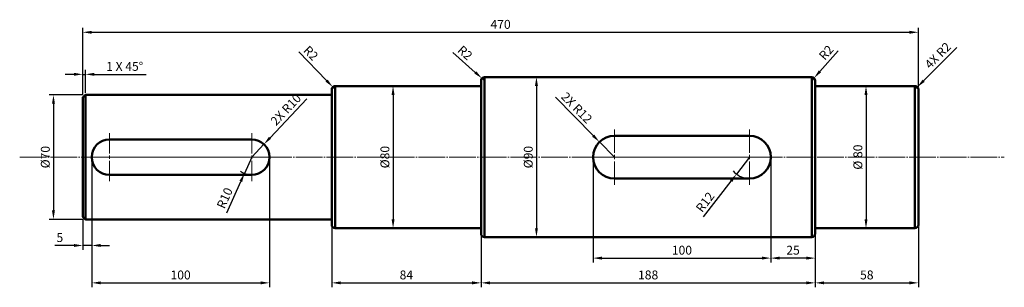
# Model space of a CAD drawing. Units: millimetres. Extents: x 186344 to 186897, y 72203 to 72353.
import ezdxf

# ---------------------------------------------------------------- set-up
doc = ezdxf.new("R2010")
doc.units = ezdxf.units.MM
doc.linetypes.add('HIDDENX2', pattern=[19.05, 12.7, -6.35])
doc.linetypes.add('JIS_08_15', pattern=[17.25, 15, -0.75, 0.75, -0.75])
doc.layers.get('Defpoints').update_dxf_attribs({"color": 3, "linetype": 'HIDDENX2'})
for name, color, linetype, lineweight in [('M-CNTR', 1, 'JIS_08_15', 18), ('M-DIMS', 4, 'Continuous', 25), ('M-OUTL', 7, 'Continuous', 50)]:
    doc.layers.add(name, color=color, linetype=linetype, lineweight=lineweight)
doc.styles.add('Annotative', font='arial.ttf')
doc.styles.get("Standard").update_dxf_attribs({"font": 'arial.ttf'})
doc.dimstyles.new('ISO-25', dxfattribs={"dimscale": 2, "dimtxt": 2.5, "dimasz": 2.5, "dimexe": 1.25, "dimexo": 0.625, "dimtad": 1, "dimtxsty": 'Standard', "dimcen": 2.5, "dimadec": 0, "dimazin": 0, "dimtfac": 1, "dimtmove": 0, "dimatfit": 3, "dimfxl": 1, "dimarcsym": 0})

# ---------------------------------------------------------------- blocks, each defined once
blk = doc.blocks.new('*U1')
at = {"layer": 'M-CNTR', "color": 0, "transparency": 16777216}
for p, q in [((0, 2.4), (0, 15.5)), ((-15.5, 0), (-2.4, 0)), ((2.4, 0), (15.5, 0)), ((0, -15.5), (0, -2.4))]:
    blk.add_line(p, q, dxfattribs=at)
at = {"layer": 'M-CNTR', "color": 0, "linetype": 'Continuous', "transparency": 16777216}
for p, q in [((-1.2, 0), (1.2, 0)), ((0, -1.2), (0, 1.2))]:
    blk.add_line(p, q, dxfattribs=at)
blk = doc.blocks.new('*U2')
at = {"layer": 'M-CNTR', "color": 0, "transparency": 16777216}
for p, q in [((0, 2.4), (0, 15.5)), ((-15.5, 0), (-2.4, 0)), ((2.4, 0), (15.5, 0)), ((0, -15.5), (0, -2.4))]:
    blk.add_line(p, q, dxfattribs=at)
at = {"layer": 'M-CNTR', "color": 0, "linetype": 'Continuous', "transparency": 16777216}
for p, q in [((-1.2, 0), (1.2, 0)), ((0, -1.2), (0, 1.2))]:
    blk.add_line(p, q, dxfattribs=at)
blk = doc.blocks.new('*D10')
at = {"layer": 'Defpoints', "color": 0, "transparency": 16777216}
for p in [(186380.52, 72311.16), (186362.58, 72241.16), (186380.52, 72241.16)]:
    blk.add_point(p, dxfattribs=at)
at = {"layer": 'M-DIMS', "color": 0, "lineweight": -2, "transparency": 16777216}
for p, q in [((186379.27, 72311.16), (186360.08, 72311.16)), ((186362.58, 72306.16), (186362.58, 72246.16)), ((186379.27, 72241.16), (186360.08, 72241.16))]:
    blk.add_line(p, q, dxfattribs=at)
at = {"layer": 'M-DIMS', "color": 0, "transparency": 16777216}
for points in [[(186361.75, 72306.16), (186363.42, 72306.16), (186362.58, 72311.16)], [(186361.75, 72246.16), (186363.42, 72246.16), (186362.58, 72241.16)]]:
    blk.add_solid(points, dxfattribs=at)
at = {"layer": 'M-DIMS', "color": 0, "transparency": 16777216, "insert": (186358.64, 72276.16), "char_height": 5, "attachment_point": 5, "rotation": 90, "style": 'Annotative'}
blk.add_mtext('%%C70', dxfattribs=at)
blk = doc.blocks.new('*D11')
at = {"layer": 'Defpoints', "color": 0, "transparency": 16777216}
for p in [(186549.8, 72316.16), (186549.8, 72236.16), (186553.62, 72236.16)]:
    blk.add_point(p, dxfattribs=at)
at = {"layer": 'M-DIMS', "color": 0, "lineweight": -2, "transparency": 16777216}
for p, q in [((186551.05, 72316.16), (186556.12, 72316.16)), ((186553.62, 72311.16), (186553.62, 72241.16)), ((186551.05, 72236.16), (186556.12, 72236.16))]:
    blk.add_line(p, q, dxfattribs=at)
at = {"layer": 'M-DIMS', "color": 0, "transparency": 16777216}
for points in [[(186552.79, 72311.16), (186554.46, 72311.16), (186553.62, 72316.16)], [(186552.79, 72241.16), (186554.46, 72241.16), (186553.62, 72236.16)]]:
    blk.add_solid(points, dxfattribs=at)
at = {"layer": 'M-DIMS', "color": 0, "transparency": 16777216, "insert": (186549.68, 72276.16), "char_height": 5, "attachment_point": 5, "rotation": 90, "style": 'Annotative'}
blk.add_mtext('%%C80', dxfattribs=at)
blk = doc.blocks.new('*D12')
at = {"layer": 'Defpoints', "color": 0, "transparency": 16777216}
for p in [(186639.08, 72321.16), (186634.27, 72231.16), (186639.08, 72231.16)]:
    blk.add_point(p, dxfattribs=at)
at = {"layer": 'M-DIMS', "color": 0, "lineweight": -2, "transparency": 16777216}
for p, q in [((186637.83, 72321.16), (186631.77, 72321.16)), ((186634.27, 72316.16), (186634.27, 72236.16)), ((186637.83, 72231.16), (186631.77, 72231.16))]:
    blk.add_line(p, q, dxfattribs=at)
at = {"layer": 'M-DIMS', "color": 0, "transparency": 16777216}
for points in [[(186633.43, 72316.16), (186635.1, 72316.16), (186634.27, 72321.16)], [(186633.43, 72236.16), (186635.1, 72236.16), (186634.27, 72231.16)]]:
    blk.add_solid(points, dxfattribs=at)
at = {"layer": 'M-DIMS', "color": 0, "transparency": 16777216, "insert": (186630.32, 72276.16), "char_height": 5, "attachment_point": 5, "rotation": 90, "style": 'Annotative'}
blk.add_mtext('%%C90', dxfattribs=at)
blk = doc.blocks.new('*D13')
at = {"layer": 'Defpoints', "color": 0, "transparency": 16777216}
for p in [(186813.24, 72316.16), (186813.24, 72236.16), (186819.65, 72236.16)]:
    blk.add_point(p, dxfattribs=at)
at = {"layer": 'M-DIMS', "color": 0, "lineweight": -2, "transparency": 16777216}
for p, q in [((186814.49, 72316.16), (186822.15, 72316.16)), ((186819.65, 72311.16), (186819.65, 72241.16)), ((186814.49, 72236.16), (186822.15, 72236.16))]:
    blk.add_line(p, q, dxfattribs=at)
at = {"layer": 'M-DIMS', "color": 0, "transparency": 16777216}
for points in [[(186818.82, 72311.16), (186820.49, 72311.16), (186819.65, 72316.16)], [(186818.82, 72241.16), (186820.49, 72241.16), (186819.65, 72236.16)]]:
    blk.add_solid(points, dxfattribs=at)
at = {"layer": 'M-DIMS', "color": 0, "transparency": 16777216, "insert": (186815.71, 72276.16), "char_height": 5, "attachment_point": 5, "rotation": 90, "style": 'Annotative'}
blk.add_mtext('%%C 80', dxfattribs=at)
blk = doc.blocks.new('*D14')
at = {"layer": 'Defpoints', "color": 0, "transparency": 16777216}
for p in [(186380.52, 72322.73), (186379.1, 72309.75), (186380.52, 72311.16)]:
    blk.add_point(p, dxfattribs=at)
at = {"layer": 'M-DIMS', "color": 0, "lineweight": -2, "transparency": 16777216}
for p, q in [((186374.1, 72322.73), (186369.1, 72322.73)), ((186379.1, 72311), (186379.1, 72325.23)), ((186379.1, 72322.73), (186380.52, 72322.73)), ((186380.52, 72312.41), (186380.52, 72325.23)), ((186385.52, 72322.73), (186414.78, 72322.73))]:
    blk.add_line(p, q, dxfattribs=at)
at = {"layer": 'M-DIMS', "color": 0, "transparency": 16777216}
for points in [[(186374.1, 72323.57), (186374.1, 72321.9), (186379.1, 72322.73)], [(186385.52, 72323.57), (186385.52, 72321.9), (186380.52, 72322.73)]]:
    blk.add_solid(points, dxfattribs=at)
at = {"layer": 'M-DIMS', "color": 0, "transparency": 16777216, "insert": (186402.65, 72326.54), "char_height": 5, "attachment_point": 5, "style": 'Annotative'}
blk.add_mtext('1 X 45%%D', dxfattribs=at)
blk = doc.blocks.new('*U3')
at = {"layer": 'M-CNTR', "color": 0, "transparency": 16777216}
for p, q in [((0, 2), (0, 13.5)), ((-13.5, 0), (-2, 0)), ((2, 0), (13.5, 0)), ((0, -13.5), (0, -2))]:
    blk.add_line(p, q, dxfattribs=at)
at = {"layer": 'M-CNTR', "color": 0, "linetype": 'Continuous', "transparency": 16777216}
for p, q in [((-1, 0), (1, 0)), ((0, -1), (0, 1))]:
    blk.add_line(p, q, dxfattribs=at)
blk = doc.blocks.new('*U4')
at = {"layer": 'M-CNTR', "color": 0, "transparency": 16777216}
for p, q in [((0, 2), (0, 13.5)), ((-13.5, 0), (-2, 0)), ((2, 0), (13.5, 0)), ((0, -13.5), (0, -2))]:
    blk.add_line(p, q, dxfattribs=at)
at = {"layer": 'M-CNTR', "color": 0, "linetype": 'Continuous', "transparency": 16777216}
for p, q in [((-1, 0), (1, 0)), ((0, -1), (0, 1))]:
    blk.add_line(p, q, dxfattribs=at)
blk = doc.blocks.new('*D5')
at = {"layer": 'Defpoints', "color": 0, "transparency": 16777216}
for p in [(186474.1, 72276.16), (186470.01, 72267.03)]:
    blk.add_point(p, dxfattribs=at)
at = {"layer": 'M-DIMS', "color": 0, "lineweight": -2, "transparency": 16777216}
for p, q in [((186474.1, 72276.16), (186470.01, 72267.03)), ((186460.02, 72244.74), (186467.97, 72262.47))]:
    blk.add_line(p, q, dxfattribs=at)
blk.add_arc((186474.1, 72276.16), 10, 231.532, 262.838, dxfattribs=at)
at = {"layer": 'M-DIMS', "color": 0, "transparency": 16777216}
blk.add_solid([(186467.21, 72262.81), (186468.73, 72262.13), (186470.01, 72267.03)], dxfattribs=at)
at = {"layer": 'M-DIMS', "color": 0, "transparency": 16777216, "insert": (186459.5, 72252.88), "char_height": 5, "attachment_point": 5, "rotation": 65.856, "style": 'Annotative'}
blk.add_mtext('R10', dxfattribs=at)
blk = doc.blocks.new('*D6')
at = {"layer": 'Defpoints', "color": 0, "transparency": 16777216}
for p in [(186754.1, 72276.16), (186746.79, 72266.64)]:
    blk.add_point(p, dxfattribs=at)
at = {"layer": 'M-DIMS', "color": 0, "lineweight": -2, "transparency": 16777216}
for p, q in [((186754.1, 72276.16), (186746.79, 72266.64)), ((186728.23, 72242.49), (186743.74, 72262.68))]:
    blk.add_line(p, q, dxfattribs=at)
blk.add_arc((186754.1, 72276.16), 12, 220.5254, 264.0317, dxfattribs=at)
at = {"layer": 'M-DIMS', "color": 0, "transparency": 16777216}
blk.add_solid([(186743.08, 72263.19), (186744.41, 72262.17), (186746.79, 72266.64)], dxfattribs=at)
at = {"layer": 'M-DIMS', "color": 0, "transparency": 16777216, "insert": (186729.63, 72250.48), "char_height": 5, "attachment_point": 5, "rotation": 52.462, "style": 'Annotative'}
blk.add_mtext('R12', dxfattribs=at)
blk = doc.blocks.new('*D7')
at = {"layer": 'Defpoints', "color": 0, "transparency": 16777216}
for p in [(186519.71, 72315.6), (186521.1, 72314.16)]:
    blk.add_point(p, dxfattribs=at)
at = {"layer": 'M-DIMS', "color": 0, "lineweight": -2, "transparency": 16777216}
for p, q in [((186500.56, 72335.36), (186516.23, 72319.19)), ((186521.1, 72314.16), (186519.71, 72315.6))]:
    blk.add_line(p, q, dxfattribs=at)
at = {"layer": 'M-DIMS', "color": 0, "transparency": 16777216}
blk.add_solid([(186516.83, 72319.77), (186515.63, 72318.61), (186519.71, 72315.6)], dxfattribs=at)
at = {"layer": 'M-DIMS', "color": 0, "transparency": 16777216, "insert": (186506.92, 72334.2), "char_height": 5, "attachment_point": 5, "rotation": 314.0907, "style": 'Annotative'}
blk.add_mtext('R2', dxfattribs=at)
blk = doc.blocks.new('*D8')
at = {"layer": 'Defpoints', "color": 0, "transparency": 16777216}
for p in [(186603.61, 72320.49), (186605.1, 72319.16)]:
    blk.add_point(p, dxfattribs=at)
at = {"layer": 'M-DIMS', "color": 0, "lineweight": -2, "transparency": 16777216}
for p, q in [((186587.26, 72335.07), (186599.88, 72323.82)), ((186605.1, 72319.16), (186603.61, 72320.49))]:
    blk.add_line(p, q, dxfattribs=at)
at = {"layer": 'M-DIMS', "color": 0, "transparency": 16777216}
blk.add_solid([(186600.43, 72324.44), (186599.32, 72323.2), (186603.61, 72320.49)], dxfattribs=at)
at = {"layer": 'M-DIMS', "color": 0, "transparency": 16777216, "insert": (186593.68, 72334.38), "char_height": 5, "attachment_point": 5, "rotation": 318.2831, "style": 'Annotative'}
blk.add_mtext('R2', dxfattribs=at)
blk = doc.blocks.new('*D9')
at = {"layer": 'Defpoints', "color": 0, "transparency": 16777216}
for p in [(186789.1, 72319.16), (186790.43, 72320.66)]:
    blk.add_point(p, dxfattribs=at)
at = {"layer": 'M-DIMS', "color": 0, "lineweight": -2, "transparency": 16777216}
for p, q in [((186804.03, 72336.01), (186793.74, 72324.4)), ((186789.1, 72319.16), (186790.43, 72320.66))]:
    blk.add_line(p, q, dxfattribs=at)
at = {"layer": 'M-DIMS', "color": 0, "transparency": 16777216}
blk.add_solid([(186793.12, 72324.95), (186794.37, 72323.85), (186790.43, 72320.66)], dxfattribs=at)
at = {"layer": 'M-DIMS', "color": 0, "transparency": 16777216, "insert": (186797.73, 72334.57), "char_height": 5, "attachment_point": 5, "rotation": 48.4635, "style": 'Annotative'}
blk.add_mtext('R2', dxfattribs=at)
blk = doc.blocks.new('*D15')
at = {"layer": 'Defpoints', "color": 0, "transparency": 16777216}
for p in [(186384.1, 72276.16), (186379.1, 72242.57), (186379.1, 72226.46)]:
    blk.add_point(p, dxfattribs=at)
at = {"layer": 'M-DIMS', "color": 0, "lineweight": -2, "transparency": 16777216}
for p, q in [((186384.1, 72274.91), (186384.1, 72223.96)), ((186379.1, 72241.32), (186379.1, 72223.96)), ((186374.1, 72226.46), (186363.29, 72226.46)), ((186384.1, 72226.46), (186379.1, 72226.46)), ((186389.1, 72226.46), (186394.1, 72226.46))]:
    blk.add_line(p, q, dxfattribs=at)
at = {"layer": 'M-DIMS', "color": 0, "transparency": 16777216}
for points in [[(186374.1, 72227.3), (186374.1, 72225.63), (186379.1, 72226.46)], [(186389.1, 72227.3), (186389.1, 72225.63), (186384.1, 72226.46)]]:
    blk.add_solid(points, dxfattribs=at)
at = {"layer": 'M-DIMS', "color": 0, "transparency": 16777216, "insert": (186366.19, 72230.26), "char_height": 5, "attachment_point": 5, "style": 'Annotative'}
blk.add_mtext('5', dxfattribs=at)
blk = doc.blocks.new('*D16')
at = {"layer": 'Defpoints', "color": 0, "transparency": 16777216}
for p in [(186384.1, 72276.16), (186484.1, 72276.16), (186484.1, 72205.43)]:
    blk.add_point(p, dxfattribs=at)
at = {"layer": 'M-DIMS', "color": 0, "lineweight": -2, "transparency": 16777216}
for p, q in [((186384.1, 72274.91), (186384.1, 72202.93)), ((186484.1, 72274.91), (186484.1, 72202.93)), ((186389.1, 72205.43), (186479.1, 72205.43))]:
    blk.add_line(p, q, dxfattribs=at)
at = {"layer": 'M-DIMS', "color": 0, "transparency": 16777216}
for points in [[(186389.1, 72206.26), (186389.1, 72204.59), (186384.1, 72205.43)], [(186479.1, 72206.26), (186479.1, 72204.59), (186484.1, 72205.43)]]:
    blk.add_solid(points, dxfattribs=at)
at = {"layer": 'M-DIMS', "color": 0, "transparency": 16777216, "insert": (186434.1, 72209.23), "char_height": 5, "attachment_point": 5, "style": 'Annotative'}
blk.add_mtext('100', dxfattribs=at)
blk = doc.blocks.new('*D17')
at = {"layer": 'Defpoints', "color": 0, "transparency": 16777216}
for p in [(186519.1, 72241.16), (186603.1, 72236.16), (186603.1, 72205.43)]:
    blk.add_point(p, dxfattribs=at)
at = {"layer": 'M-DIMS', "color": 0, "lineweight": -2, "transparency": 16777216}
for p, q in [((186519.1, 72239.91), (186519.1, 72202.93)), ((186603.1, 72234.91), (186603.1, 72202.93)), ((186524.1, 72205.43), (186598.1, 72205.43))]:
    blk.add_line(p, q, dxfattribs=at)
at = {"layer": 'M-DIMS', "color": 0, "transparency": 16777216}
for points in [[(186524.1, 72206.26), (186524.1, 72204.59), (186519.1, 72205.43)], [(186598.1, 72206.26), (186598.1, 72204.59), (186603.1, 72205.43)]]:
    blk.add_solid(points, dxfattribs=at)
at = {"layer": 'M-DIMS', "color": 0, "transparency": 16777216, "insert": (186561.1, 72209.23), "char_height": 5, "attachment_point": 5, "style": 'Annotative'}
blk.add_mtext('84', dxfattribs=at)
blk = doc.blocks.new('*D18')
at = {"layer": 'Defpoints', "color": 0, "transparency": 16777216}
for p in [(186603.1, 72236.16), (186791.1, 72236.16), (186791.1, 72205.43)]:
    blk.add_point(p, dxfattribs=at)
at = {"layer": 'M-DIMS', "color": 0, "lineweight": -2, "transparency": 16777216}
for p, q in [((186603.1, 72234.91), (186603.1, 72202.93)), ((186791.1, 72234.91), (186791.1, 72202.93)), ((186608.1, 72205.43), (186786.1, 72205.43))]:
    blk.add_line(p, q, dxfattribs=at)
at = {"layer": 'M-DIMS', "color": 0, "transparency": 16777216}
for points in [[(186608.1, 72206.26), (186608.1, 72204.59), (186603.1, 72205.43)], [(186786.1, 72206.26), (186786.1, 72204.59), (186791.1, 72205.43)]]:
    blk.add_solid(points, dxfattribs=at)
at = {"layer": 'M-DIMS', "color": 0, "transparency": 16777216, "insert": (186697.1, 72209.23), "char_height": 5, "attachment_point": 5, "style": 'Annotative'}
blk.add_mtext('188', dxfattribs=at)
blk = doc.blocks.new('*D19')
at = {"layer": 'Defpoints', "color": 0, "transparency": 16777216}
for p in [(186791.1, 72236.16), (186849.1, 72238.16), (186849.1, 72205.43)]:
    blk.add_point(p, dxfattribs=at)
at = {"layer": 'M-DIMS', "color": 0, "lineweight": -2, "transparency": 16777216}
for p, q in [((186791.1, 72234.91), (186791.1, 72202.93)), ((186849.1, 72236.91), (186849.1, 72202.93)), ((186796.1, 72205.43), (186844.1, 72205.43))]:
    blk.add_line(p, q, dxfattribs=at)
at = {"layer": 'M-DIMS', "color": 0, "transparency": 16777216}
for points in [[(186796.1, 72206.26), (186796.1, 72204.59), (186791.1, 72205.43)], [(186844.1, 72206.26), (186844.1, 72204.59), (186849.1, 72205.43)]]:
    blk.add_solid(points, dxfattribs=at)
at = {"layer": 'M-DIMS', "color": 0, "transparency": 16777216, "insert": (186820.1, 72209.23), "char_height": 5, "attachment_point": 5, "style": 'Annotative'}
blk.add_mtext('58', dxfattribs=at)
blk = doc.blocks.new('*D20')
at = {"layer": 'Defpoints', "color": 0, "transparency": 16777216}
for p in [(186766.1, 72276.16), (186791.1, 72236.16), (186766.1, 72219.35)]:
    blk.add_point(p, dxfattribs=at)
at = {"layer": 'M-DIMS', "color": 0, "lineweight": -2, "transparency": 16777216}
for p, q in [((186766.1, 72274.91), (186766.1, 72216.85)), ((186791.1, 72234.91), (186791.1, 72216.85)), ((186786.1, 72219.35), (186771.1, 72219.35))]:
    blk.add_line(p, q, dxfattribs=at)
at = {"layer": 'M-DIMS', "color": 0, "transparency": 16777216}
for points in [[(186771.1, 72220.19), (186771.1, 72218.52), (186766.1, 72219.35)], [(186786.1, 72220.19), (186786.1, 72218.52), (186791.1, 72219.35)]]:
    blk.add_solid(points, dxfattribs=at)
at = {"layer": 'M-DIMS', "color": 0, "transparency": 16777216, "insert": (186778.6, 72223.16), "char_height": 5, "attachment_point": 5, "style": 'Annotative'}
blk.add_mtext('25', dxfattribs=at)
blk = doc.blocks.new('*D21')
at = {"layer": 'Defpoints', "color": 0, "transparency": 16777216}
for p in [(186666.1, 72276.16), (186766.1, 72276.16), (186766.1, 72219.35)]:
    blk.add_point(p, dxfattribs=at)
at = {"layer": 'M-DIMS', "color": 0, "lineweight": -2, "transparency": 16777216}
for p, q in [((186666.1, 72274.91), (186666.1, 72216.85)), ((186766.1, 72274.91), (186766.1, 72216.85)), ((186671.1, 72219.35), (186761.1, 72219.35))]:
    blk.add_line(p, q, dxfattribs=at)
at = {"layer": 'M-DIMS', "color": 0, "transparency": 16777216}
for points in [[(186671.1, 72220.19), (186671.1, 72218.52), (186666.1, 72219.35)], [(186761.1, 72220.19), (186761.1, 72218.52), (186766.1, 72219.35)]]:
    blk.add_solid(points, dxfattribs=at)
at = {"layer": 'M-DIMS', "color": 0, "transparency": 16777216, "insert": (186716.1, 72223.16), "char_height": 5, "attachment_point": 5, "style": 'Annotative'}
blk.add_mtext('100', dxfattribs=at)
blk = doc.blocks.new('*D22')
at = {"layer": 'Defpoints', "color": 0, "transparency": 16777216}
for p in [(186849.1, 72346.39), (186849.1, 72314.16), (186379.1, 72309.75)]:
    blk.add_point(p, dxfattribs=at)
at = {"layer": 'M-DIMS', "color": 0, "lineweight": -2, "transparency": 16777216}
for p, q in [((186379.1, 72311), (186379.1, 72348.89)), ((186384.1, 72346.39), (186844.1, 72346.39)), ((186849.1, 72315.41), (186849.1, 72348.89))]:
    blk.add_line(p, q, dxfattribs=at)
at = {"layer": 'M-DIMS', "color": 0, "transparency": 16777216}
for points in [[(186384.1, 72347.22), (186384.1, 72345.55), (186379.1, 72346.39)], [(186844.1, 72347.22), (186844.1, 72345.55), (186849.1, 72346.39)]]:
    blk.add_solid(points, dxfattribs=at)
at = {"layer": 'M-DIMS', "color": 0, "transparency": 16777216, "insert": (186614.1, 72350.19), "char_height": 5, "attachment_point": 5, "style": 'Annotative'}
blk.add_mtext('470', dxfattribs=at)
blk = doc.blocks.new('*D23')
at = {"layer": 'Defpoints', "color": 0, "transparency": 16777216}
for p in [(186480.97, 72283.42), (186474.1, 72276.16)]:
    blk.add_point(p, dxfattribs=at)
at = {"layer": 'M-DIMS', "color": 0, "lineweight": -2, "transparency": 16777216}
for p, q in [((186505.2, 72309.04), (186484.41, 72287.06)), ((186474.1, 72276.16), (186480.97, 72283.42))]:
    blk.add_line(p, q, dxfattribs=at)
at = {"layer": 'M-DIMS', "color": 0, "transparency": 16777216}
blk.add_solid([(186483.8, 72287.63), (186485.02, 72286.48), (186480.97, 72283.42)], dxfattribs=at)
at = {"layer": 'M-DIMS', "color": 0, "transparency": 16777216, "insert": (186493.76, 72302.48), "char_height": 5, "attachment_point": 5, "rotation": 46.5937}
blk.add_mtext('2X R10', dxfattribs=at)
blk = doc.blocks.new('*D24')
at = {"layer": 'Defpoints', "color": 0, "transparency": 16777216}
for p in [(186669.68, 72284.71), (186678.1, 72276.16)]:
    blk.add_point(p, dxfattribs=at)
at = {"layer": 'M-DIMS', "color": 0, "lineweight": -2, "transparency": 16777216}
for p, q in [((186644.96, 72309.8), (186666.17, 72288.27)), ((186678.1, 72276.16), (186669.68, 72284.71))]:
    blk.add_line(p, q, dxfattribs=at)
at = {"layer": 'M-DIMS', "color": 0, "transparency": 16777216}
blk.add_solid([(186666.77, 72288.85), (186665.58, 72287.68), (186669.68, 72284.71)], dxfattribs=at)
at = {"layer": 'M-DIMS', "color": 0, "transparency": 16777216, "insert": (186656.49, 72303.46), "char_height": 5, "attachment_point": 5, "rotation": 314.5722}
blk.add_mtext('2X R12', dxfattribs=at)
blk = doc.blocks.new('*D25')
at = {"layer": 'Defpoints', "color": 0, "transparency": 16777216}
for p in [(186847.1, 72314.16), (186848.52, 72315.57)]:
    blk.add_point(p, dxfattribs=at)
at = {"layer": 'M-DIMS', "color": 0, "lineweight": -2, "transparency": 16777216}
for p, q in [((186870.76, 72337.82), (186852.05, 72319.11)), ((186847.1, 72314.16), (186848.52, 72315.57))]:
    blk.add_line(p, q, dxfattribs=at)
at = {"layer": 'M-DIMS', "color": 0, "transparency": 16777216}
blk.add_solid([(186851.46, 72319.7), (186852.64, 72318.52), (186848.52, 72315.57)], dxfattribs=at)
at = {"layer": 'M-DIMS', "color": 0, "transparency": 16777216, "insert": (186860.51, 72332.89), "char_height": 5, "attachment_point": 5, "rotation": 45.0017}
blk.add_mtext('4X R2', dxfattribs=at)

msp = doc.modelspace()

# ---------------------------------------------------------------- linework, layer by layer
at = {"layer": 'M-CNTR'}
for p, q in [((186343.59, 72276.159), (186897.446, 72276.159)), ((186384.102, 72276.159), (186484.102, 72276.159)), ((186659.11, 72276.159), (186771.465, 72276.159))]:
    msp.add_line(p, q, dxfattribs=at)
at = {"layer": 'M-OUTL'}
for p, q in [((186603.102, 72233.159), (186603.102, 72319.159)), ((186605.102, 72321.159), (186789.102, 72321.159)), ((186605.102, 72231.159), (186605.102, 72321.159)), ((186789.102, 72321.159), (186789.102, 72231.159)), ((186789.102, 72231.159), (186789.102, 72321.159)), ((186791.102, 72233.159), (186791.102, 72319.159)), ((186519.102, 72238.159), (186519.102, 72314.159)), ((186521.102, 72316.159), (186603.102, 72316.159)), ((186521.102, 72236.159), (186521.102, 72316.159)), ((186603.102, 72316.159), (186603.102, 72236.159)), ((186791.102, 72316.159), (186847.102, 72316.159)), ((186791.102, 72236.159), (186791.102, 72316.159)), ((186847.102, 72316.159), (186847.102, 72236.159)), ((186849.102, 72314.159), (186849.102, 72238.159)), ((186394.102, 72286.159), (186474.102, 72286.159)), ((186678.102, 72288.159), (186754.102, 72288.159)), ((186474.102, 72266.159), (186394.102, 72266.159)), ((186678.102, 72264.159), (186754.102, 72264.159)), ((186603.102, 72236.159), (186521.102, 72236.159)), ((186847.102, 72236.159), (186791.102, 72236.159)), ((186789.102, 72231.159), (186605.102, 72231.159))]:
    msp.add_line(p, q, dxfattribs=at)
msp.add_lwpolyline([(186380.517, 72241.159), (186379.102, 72242.573), (186379.102, 72309.745), (186380.517, 72311.159), (186380.517, 72241.159), (186519.102, 72241.159), (186519.102, 72311.159), (186380.517, 72311.159)], dxfattribs=at)
for centre, radius, start, end in [((186605.102, 72319.159), 2, 90, 180), ((186789.102, 72319.159), 2, 0, 90), ((186521.102, 72314.159), 2, 90, 180), ((186847.102, 72314.159), 2, 0, 90), ((186394.102, 72276.159), 10, 90, 270), ((186474.102, 72276.159), 10, 270, 90), ((186678.102, 72276.159), 12, 90, 270), ((186754.102, 72276.159), 12, 270, 90), ((186521.102, 72238.159), 2, 180, 270), ((186847.102, 72238.159), 2, 270, 0), ((186605.102, 72233.159), 2, 180, 270), ((186789.102, 72233.159), 2, 270, 0)]:
    msp.add_arc(centre, radius, start, end, dxfattribs=at)

# ---------------------------------------------------------------- block references
at = {"layer": 'M-CNTR'}
for name, p in [('*U3', (186394.102, 72276.159)), ('*U4', (186474.102, 72276.159)), ('*U1', (186678.102, 72276.159)), ('*U2', (186754.102, 72276.159))]:
    msp.add_blockref(name, p, dxfattribs=at)

# ---------------------------------------------------------------- dimensions: what is measured, and where the dimension line sits
at = {"layer": 'M-DIMS'}
for base, p1, p2, picture, middle in [((186849.102, 72346.385), (186379.102, 72309.745), (186849.102, 72314.159), '*D22', (186614.102, 72350.188)), ((186379.102, 72226.463), (186384.102, 72276.159), (186379.102, 72242.573), '*D15', (186366.195, 72230.256)), ((186484.102, 72205.426), (186384.102, 72276.159), (186484.102, 72276.159), '*D16', (186434.102, 72209.229)), ((186766.102, 72219.354), (186666.102, 72276.159), (186766.102, 72276.159), '*D21', (186716.102, 72223.157)), ((186766.102, 72219.354), (186791.102, 72236.159), (186766.102, 72276.159), '*D20', (186778.602, 72223.157)), ((186603.102, 72205.426), (186519.102, 72241.159), (186603.102, 72236.159), '*D17', (186561.102, 72209.229)), ((186791.102, 72205.426), (186603.102, 72236.159), (186791.102, 72236.159), '*D18', (186697.102, 72209.229)), ((186849.102, 72205.426), (186791.102, 72236.159), (186849.102, 72238.159), '*D19', (186820.102, 72209.229))]:
    dim = msp.add_linear_dim(base=base, p1=p1, p2=p2, dimstyle='ISO-25', override={"dimtxsty": 'Annotative', "dimclrd": 0, "dimclre": 0, "dimclrt": 0}, dxfattribs=at)
    dim.commit()
    dim.dimension.update_dxf_attribs({"geometry": picture, "text_midpoint": middle})
for center, mpoint, picture, middle in [((186521.102, 72314.159), (186519.711, 72315.596), '*D7', (186504.219, 72331.587)), ((186605.102, 72319.159), (186603.609, 72320.49), '*D8', (186591.18, 72331.571)), ((186754.102, 72276.159), (186746.791, 72266.644), '*D6', (186732.614, 72248.193))]:
    dim = msp.add_radius_dim(center=center, mpoint=mpoint, dimstyle='ISO-25', override={"dimtxsty": 'Annotative', "dimclrd": 0, "dimclre": 0, "dimclrt": 0}, dxfattribs=at)
    dim.commit()
    dim.dimension.update_dxf_attribs({"geometry": picture, "text_midpoint": middle, "dimtype": 164})
for center, mpoint, picture, middle in [((186789.102, 72319.159), (186790.429, 72320.656), '*D9', (186797.73, 72334.569)), ((186474.102, 72276.159), (186470.012, 72267.034), '*D5', (186459.5, 72252.88))]:
    dim = msp.add_radius_dim(center=center, mpoint=mpoint, dimstyle='ISO-25', override={"dimtxsty": 'Annotative', "dimclrd": 0, "dimclre": 0, "dimclrt": 0}, dxfattribs=at)
    dim.commit()
    dim.dimension.update_dxf_attribs({"geometry": picture, "text_midpoint": middle})
for center, mpoint, text, picture, middle in [((186847.102, 72314.159), (186848.516, 72315.573), '4X <>', '*D25', (186860.513, 72332.891)), ((186474.102, 72276.159), (186480.974, 72283.424), '2X <>', '*D23', (186493.762, 72302.478)), ((186678.102, 72276.159), (186669.681, 72284.708), '2X <>', '*D24', (186656.491, 72303.456))]:
    dim = msp.add_radius_dim(center=center, mpoint=mpoint, text=text, dimstyle='ISO-25', override={"dimdec": 0, "dimlfac": 1, "dimrnd": 0, "dimzin": 0, "dimdsep": 46, "dimlunit": 2}, dxfattribs=at)
    dim.commit()
    dim.dimension.update_dxf_attribs({"geometry": picture, "text_midpoint": middle})
dim = msp.add_linear_dim(base=(186380.517, 72322.734), p1=(186379.102, 72309.745), p2=(186380.517, 72311.159), text='<> X 45%%D', dimstyle='ISO-25', override={"dimdec": 0, "dimtxsty": 'Annotative', "dimclrd": 0, "dimclre": 0, "dimclrt": 0}, dxfattribs=at)
dim.commit()
dim.dimension.update_dxf_attribs({"geometry": '*D14', "text_midpoint": (186402.648, 72326.537)})
for base, p1, p2, text, picture, middle in [((186634.267, 72231.159), (186639.079, 72321.159), (186639.079, 72231.159), '%%C<>', '*D12', (186630.325, 72276.159)), ((186553.622, 72236.159), (186549.795, 72316.159), (186549.795, 72236.159), '%%C<>', '*D11', (186549.679, 72276.159)), ((186819.654, 72236.159), (186813.243, 72316.159), (186813.243, 72236.159), '%%C <>', '*D13', (186815.712, 72276.159)), ((186362.583, 72241.159), (186380.517, 72311.159), (186380.517, 72241.159), '%%C<>', '*D10', (186358.64, 72276.159))]:
    dim = msp.add_linear_dim(base=base, p1=p1, p2=p2, angle=90, text=text, dimstyle='ISO-25', override={"dimtxsty": 'Annotative', "dimclrd": 0, "dimclre": 0, "dimclrt": 0}, dxfattribs=at)
    dim.commit()
    dim.dimension.update_dxf_attribs({"geometry": picture, "text_midpoint": middle})

doc.saveas('drawing.dxf')
